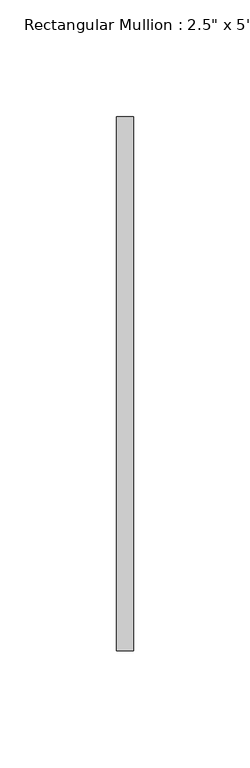
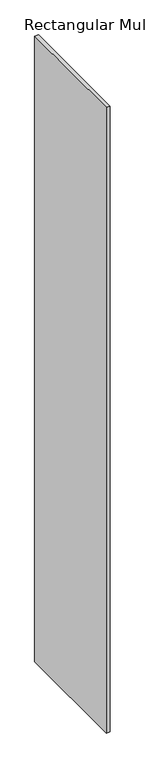
"""IFC4 building model written with IfcOpenShell, lengths in millimetres: member geometry."""

from ifc_helpers import new_model, si_unit, frame, origin, place, context, project, spatial, polyline, outline, extrude, source, transform, mapped, element, save


def member_81a97153(model_context):
    return source(origin(), model_context, "Body", "SweptSolid", [
        extrude(outline(polyline([(0.0, 114.3), (0.0, -114.3), (-7.239, -114.3), (-7.239, 114.3), (0.0, 114.3)])), frame((0.0, 0.0, -1219.2), z_axis=(0.0, 0.0, 1.0), x_axis=(1.0, 0.0, 0.0)), (0.0, 0.0, 1.0), 1219.2),
    ])


if __name__ == "__main__":
    model = new_model("IFC4")
    model_context = context("Model", 3, world=origin())
    ifc_project = project(units=[si_unit("LENGTHUNIT", "METRE", prefix="MILLI")], contexts=[model_context])
    site = spatial("IfcSite", under=ifc_project)
    building = spatial("IfcBuilding", under=site)
    placement = place(None, origin())
    member_shape = member_81a97153(model_context)
    element("IfcMember", 1, ObjectType="Rectangular Mullion : 2.5\" x 5\" rectangular", at=placement, inside=building, context=model_context, shape_type="MappedRepresentation", body=[
        mapped(member_shape, transform((0.0, 0.0, 0.0), x_axis=(1.0, 0.0, 0.0), y_axis=(0.0, 1.0, 0.0), z_axis=(0.0, 0.0, 1.0))),
    ])
    save(model, "model.ifc")

# Revit data of these elements
# Type "Rectangular Mullion : 2.5\" x 5\" rectangular"
#   built-in parameter 1007304 = 0.75 (stored number, unit not read)
#   built-in parameter 1007301 = 0.011875 (stored number, unit not read)
#   built-in parameter 1007300 = 0.011875 (stored number, unit not read)
# Element 1 (IfcMember, "Rectangular Mullion : 2.5\" x 5\" rectangular")
#   Materials on its faces: "WINDOW GLASS MATERIAL"
# Materials
#   "WINDOW GLASS MATERIAL": class "Generic", colour RGB 120 120 120, transparency 0, Cost = 0
